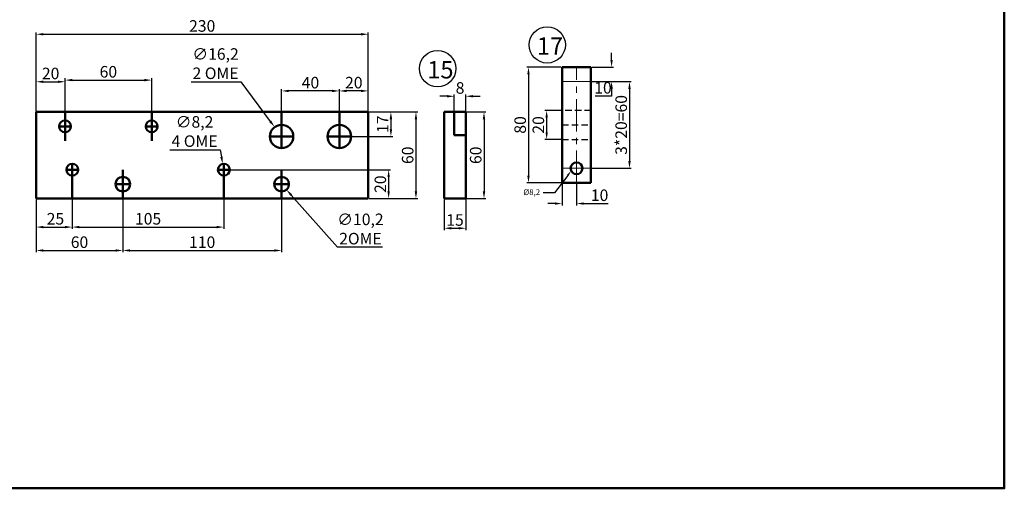
# Model space of a CAD drawing. Units: millimetres. Extents: x -749 to 333, y -22 to 680.
# Tile 3 of 4: x -349 to 333, y -22 to 302. Entities that reach past the tile are written whole.
import ezdxf
from ezdxf import colors
from ezdxf.entities.mleader import LeaderData, LeaderLine
from ezdxf.math import Vec2, Vec3

# ---------------------------------------------------------------- set-up
doc = ezdxf.new("R2010")
doc.units = ezdxf.units.MM
doc.header["$LTSCALE"] = 0.7
doc.linetypes.add('CENTER', pattern=[50.8, 31.75, -6.35, 6.35, -6.35])
doc.linetypes.add('HIDDEN', pattern=[9.525, 6.35, -3.175])
for name, color, linetype, lineweight in [('M-CNTR', 1, 'CENTER', 18), ('M-DIMS', 2, 'Continuous', 25), ('M-HIDN', 4, 'HIDDEN', 25), ('M-OUTL', 7, 'Continuous', 50), ('M-TEXT', 3, 'Continuous', 25), ('M-TTLB', 7, 'Continuous', 50)]:
    doc.layers.add(name, color=color, linetype=linetype, lineweight=lineweight)
doc.styles.get("Standard").update_dxf_attribs({"font": 'arial.ttf'})
doc.dimstyles.new('ISO-25', dxfattribs={"dimtxt": 8, "dimasz": 5, "dimexe": 1.25, "dimexo": 0.625, "dimtad": 1, "dimtoh": 1, "dimtxsty": 'Standard', "dimcen": 2.5, "dimadec": 0, "dimazin": 0, "dimtfac": 1, "dimtofl": 0, "dimtmove": 0, "dimatfit": 3, "dimfxl": 1, "dimarcsym": 0})

# ---------------------------------------------------------------- blocks, each defined once
blk = doc.blocks.new('*D43')
at = {"layer": 'Defpoints', "color": 0, "transparency": 16777216}
for p in [(-107.83, 238.25), (-107.83, 178.25), (-74.76, 178.25)]:
    blk.add_point(p, dxfattribs=at)
at = {"layer": 'M-DIMS', "color": 0, "lineweight": -2, "transparency": 16777216}
for p, q in [((-107.21, 238.25), (-73.51, 238.25)), ((-74.76, 233.25), (-74.76, 183.25)), ((-107.21, 178.25), (-73.51, 178.25))]:
    blk.add_line(p, q, dxfattribs=at)
at = {"layer": 'M-DIMS', "color": 0, "transparency": 16777216}
for points in [[(-75.6, 233.25), (-73.93, 233.25), (-74.76, 238.25)], [(-75.6, 183.25), (-73.93, 183.25), (-74.76, 178.25)]]:
    blk.add_solid(points, dxfattribs=at)
at = {"layer": 'M-DIMS', "color": 0, "transparency": 16777216, "insert": (-79.47, 208.25), "char_height": 8, "attachment_point": 5, "rotation": 90}
blk.add_mtext('60', dxfattribs=at)
blk = doc.blocks.new('*D44')
at = {"layer": 'Defpoints', "color": 0, "transparency": 16777216}
for p in [(-127.83, 238.25), (-127.83, 221.25), (-92.12, 221.25)]:
    blk.add_point(p, dxfattribs=at)
at = {"layer": 'M-DIMS', "color": 0, "lineweight": -2, "transparency": 16777216}
for p, q in [((-127.21, 238.25), (-90.87, 238.25)), ((-92.12, 233.25), (-92.12, 226.25)), ((-127.21, 221.25), (-90.87, 221.25))]:
    blk.add_line(p, q, dxfattribs=at)
at = {"layer": 'M-DIMS', "color": 0, "transparency": 16777216}
for points in [[(-92.95, 233.25), (-91.28, 233.25), (-92.12, 238.25)], [(-92.95, 226.25), (-91.28, 226.25), (-92.12, 221.25)]]:
    blk.add_solid(points, dxfattribs=at)
at = {"layer": 'M-DIMS', "color": 0, "transparency": 16777216, "insert": (-96.76, 229.75), "char_height": 8, "attachment_point": 5, "rotation": 90}
blk.add_mtext('17', dxfattribs=at)
blk = doc.blocks.new('*D45')
at = {"layer": 'Defpoints', "color": 0, "transparency": 16777216}
for p in [(-207.83, 198.25), (-107.83, 178.25), (-93.69, 178.25)]:
    blk.add_point(p, dxfattribs=at)
at = {"layer": 'M-DIMS', "color": 0, "lineweight": -2, "transparency": 16777216}
for p, q in [((-207.21, 198.25), (-92.44, 198.25)), ((-93.69, 193.25), (-93.69, 183.25)), ((-107.21, 178.25), (-92.44, 178.25))]:
    blk.add_line(p, q, dxfattribs=at)
at = {"layer": 'M-DIMS', "color": 0, "transparency": 16777216}
for points in [[(-94.53, 193.25), (-92.86, 193.25), (-93.69, 198.25)], [(-94.53, 183.25), (-92.86, 183.25), (-93.69, 178.25)]]:
    blk.add_solid(points, dxfattribs=at)
at = {"layer": 'M-DIMS', "color": 0, "transparency": 16777216, "insert": (-98.4, 188.25), "char_height": 8, "attachment_point": 5, "rotation": 90}
blk.add_mtext('20', dxfattribs=at)
blk = doc.blocks.new('*D46')
at = {"layer": 'Defpoints', "color": 0, "transparency": 16777216}
for p in [(-337.83, 178.25), (-312.83, 178.25), (-312.83, 158.55)]:
    blk.add_point(p, dxfattribs=at)
at = {"layer": 'M-DIMS', "color": 0, "lineweight": -2, "transparency": 16777216}
for p, q in [((-337.83, 177.62), (-337.83, 157.3)), ((-312.83, 177.62), (-312.83, 157.3)), ((-332.83, 158.55), (-317.83, 158.55))]:
    blk.add_line(p, q, dxfattribs=at)
at = {"layer": 'M-DIMS', "color": 0, "transparency": 16777216}
for points in [[(-332.83, 159.39), (-332.83, 157.72), (-337.83, 158.55)], [(-317.83, 159.39), (-317.83, 157.72), (-312.83, 158.55)]]:
    blk.add_solid(points, dxfattribs=at)
at = {"layer": 'M-DIMS', "color": 0, "transparency": 16777216, "insert": (-324.51, 163.26), "char_height": 8, "attachment_point": 5}
blk.add_mtext('25', dxfattribs=at)
blk = doc.blocks.new('*D47')
at = {"layer": 'Defpoints', "color": 0, "transparency": 16777216}
for p in [(-337.83, 178.25), (-277.83, 178.25), (-277.83, 142.35)]:
    blk.add_point(p, dxfattribs=at)
at = {"layer": 'M-DIMS', "color": 0, "lineweight": -2, "transparency": 16777216}
for p, q in [((-337.83, 177.62), (-337.83, 141.1)), ((-277.83, 177.62), (-277.83, 141.1)), ((-332.83, 142.35), (-282.83, 142.35))]:
    blk.add_line(p, q, dxfattribs=at)
at = {"layer": 'M-DIMS', "color": 0, "transparency": 16777216}
for points in [[(-332.83, 143.18), (-332.83, 141.52), (-337.83, 142.35)], [(-282.83, 143.18), (-282.83, 141.52), (-277.83, 142.35)]]:
    blk.add_solid(points, dxfattribs=at)
at = {"layer": 'M-DIMS', "color": 0, "transparency": 16777216, "insert": (-307.83, 147.06), "char_height": 8, "attachment_point": 5}
blk.add_mtext('60', dxfattribs=at)
blk = doc.blocks.new('*D48')
at = {"layer": 'Defpoints', "color": 0, "transparency": 16777216}
for p in [(-312.83, 178.25), (-207.83, 178.25), (-207.83, 158.55)]:
    blk.add_point(p, dxfattribs=at)
at = {"layer": 'M-DIMS', "color": 0, "lineweight": -2, "transparency": 16777216}
for p, q in [((-312.83, 177.62), (-312.83, 157.3)), ((-207.83, 177.62), (-207.83, 157.3)), ((-307.83, 158.55), (-212.83, 158.55))]:
    blk.add_line(p, q, dxfattribs=at)
at = {"layer": 'M-DIMS', "color": 0, "transparency": 16777216}
for points in [[(-307.83, 159.39), (-307.83, 157.72), (-312.83, 158.55)], [(-212.83, 159.39), (-212.83, 157.72), (-207.83, 158.55)]]:
    blk.add_solid(points, dxfattribs=at)
at = {"layer": 'M-DIMS', "color": 0, "transparency": 16777216, "insert": (-260.33, 163.26), "char_height": 8, "attachment_point": 5}
blk.add_mtext('105', dxfattribs=at)
blk = doc.blocks.new('*D49')
at = {"layer": 'Defpoints', "color": 0, "transparency": 16777216}
for p in [(-277.83, 178.25), (-167.83, 178.25), (-167.83, 142.35)]:
    blk.add_point(p, dxfattribs=at)
at = {"layer": 'M-DIMS', "color": 0, "lineweight": -2, "transparency": 16777216}
for p, q in [((-277.83, 177.62), (-277.83, 141.1)), ((-167.83, 177.62), (-167.83, 141.1)), ((-272.83, 142.35), (-172.83, 142.35))]:
    blk.add_line(p, q, dxfattribs=at)
at = {"layer": 'M-DIMS', "color": 0, "transparency": 16777216}
for points in [[(-272.83, 143.18), (-272.83, 141.52), (-277.83, 142.35)], [(-172.83, 143.18), (-172.83, 141.52), (-167.83, 142.35)]]:
    blk.add_solid(points, dxfattribs=at)
at = {"layer": 'M-DIMS', "color": 0, "transparency": 16777216, "insert": (-222.83, 147.06), "char_height": 8, "attachment_point": 5}
blk.add_mtext('110', dxfattribs=at)
blk = doc.blocks.new('*D50')
at = {"layer": 'Defpoints', "color": 0, "transparency": 16777216}
for p in [(-107.83, 292.04), (-337.83, 238.25), (-107.83, 238.25)]:
    blk.add_point(p, dxfattribs=at)
at = {"layer": 'M-DIMS', "color": 0, "lineweight": -2, "transparency": 16777216}
for p, q in [((-337.83, 238.87), (-337.83, 293.29)), ((-107.83, 238.87), (-107.83, 293.29)), ((-332.83, 292.04), (-112.83, 292.04))]:
    blk.add_line(p, q, dxfattribs=at)
at = {"layer": 'M-DIMS', "color": 0, "transparency": 16777216}
for points in [[(-332.83, 292.88), (-332.83, 291.21), (-337.83, 292.04)], [(-112.83, 292.88), (-112.83, 291.21), (-107.83, 292.04)]]:
    blk.add_solid(points, dxfattribs=at)
at = {"layer": 'M-DIMS', "color": 0, "transparency": 16777216, "insert": (-222.83, 296.76), "char_height": 8, "attachment_point": 5}
blk.add_mtext('230', dxfattribs=at)
blk = doc.blocks.new('*D51')
at = {"layer": 'Defpoints', "color": 0, "transparency": 16777216}
for p in [(-317.83, 259.16), (-337.83, 238.25), (-317.83, 238.25)]:
    blk.add_point(p, dxfattribs=at)
at = {"layer": 'M-DIMS', "color": 0, "lineweight": -2, "transparency": 16777216}
for p, q in [((-337.83, 238.87), (-337.83, 260.41)), ((-317.83, 238.87), (-317.83, 260.41)), ((-332.83, 259.16), (-322.83, 259.16))]:
    blk.add_line(p, q, dxfattribs=at)
at = {"layer": 'M-DIMS', "color": 0, "transparency": 16777216}
for points in [[(-332.83, 259.99), (-332.83, 258.32), (-337.83, 259.16)], [(-322.83, 259.99), (-322.83, 258.32), (-317.83, 259.16)]]:
    blk.add_solid(points, dxfattribs=at)
at = {"layer": 'M-DIMS', "color": 0, "transparency": 16777216, "insert": (-327.83, 263.87), "char_height": 8, "attachment_point": 5}
blk.add_mtext('20', dxfattribs=at)
blk = doc.blocks.new('*D52')
at = {"layer": 'Defpoints', "color": 0, "transparency": 16777216}
for p in [(-257.83, 260.31), (-317.83, 238.25), (-257.83, 238.25)]:
    blk.add_point(p, dxfattribs=at)
at = {"layer": 'M-DIMS', "color": 0, "lineweight": -2, "transparency": 16777216}
for p, q in [((-317.83, 238.87), (-317.83, 261.56)), ((-312.83, 260.31), (-262.83, 260.31)), ((-257.83, 238.87), (-257.83, 261.56))]:
    blk.add_line(p, q, dxfattribs=at)
at = {"layer": 'M-DIMS', "color": 0, "transparency": 16777216}
for points in [[(-312.83, 261.15), (-312.83, 259.48), (-317.83, 260.31)], [(-262.83, 261.15), (-262.83, 259.48), (-257.83, 260.31)]]:
    blk.add_solid(points, dxfattribs=at)
at = {"layer": 'M-DIMS', "color": 0, "transparency": 16777216, "insert": (-287.83, 265.02), "char_height": 8, "attachment_point": 5}
blk.add_mtext('60', dxfattribs=at)
blk = doc.blocks.new('*D53')
at = {"layer": 'Defpoints', "color": 0, "transparency": 16777216}
for p in [(-127.83, 252.81), (-127.83, 238.25), (-107.83, 238.25)]:
    blk.add_point(p, dxfattribs=at)
at = {"layer": 'M-DIMS', "color": 0, "lineweight": -2, "transparency": 16777216}
for p, q in [((-127.83, 238.87), (-127.83, 254.06)), ((-112.83, 252.81), (-122.83, 252.81)), ((-107.83, 238.87), (-107.83, 254.06))]:
    blk.add_line(p, q, dxfattribs=at)
at = {"layer": 'M-DIMS', "color": 0, "transparency": 16777216}
for points in [[(-122.83, 253.64), (-122.83, 251.98), (-127.83, 252.81)], [(-112.83, 253.64), (-112.83, 251.98), (-107.83, 252.81)]]:
    blk.add_solid(points, dxfattribs=at)
at = {"layer": 'M-DIMS', "color": 0, "transparency": 16777216, "insert": (-117.83, 257.52), "char_height": 8, "attachment_point": 5}
blk.add_mtext('20', dxfattribs=at)
blk = doc.blocks.new('*D54')
at = {"layer": 'Defpoints', "color": 0, "transparency": 16777216}
for p in [(-167.83, 252.81), (-167.83, 238.25), (-127.83, 238.25)]:
    blk.add_point(p, dxfattribs=at)
at = {"layer": 'M-DIMS', "color": 0, "lineweight": -2, "transparency": 16777216}
for p, q in [((-167.83, 238.87), (-167.83, 254.06)), ((-132.83, 252.81), (-162.83, 252.81)), ((-127.83, 238.87), (-127.83, 254.06))]:
    blk.add_line(p, q, dxfattribs=at)
at = {"layer": 'M-DIMS', "color": 0, "transparency": 16777216}
for points in [[(-162.83, 253.64), (-162.83, 251.98), (-167.83, 252.81)], [(-132.83, 253.64), (-132.83, 251.98), (-127.83, 252.81)]]:
    blk.add_solid(points, dxfattribs=at)
at = {"layer": 'M-DIMS', "color": 0, "transparency": 16777216, "insert": (-147.83, 257.52), "char_height": 8, "attachment_point": 5}
blk.add_mtext('40', dxfattribs=at)
blk = doc.blocks.new('*D55')
at = {"layer": 'Defpoints', "color": 0, "transparency": 16777216}
for p in [(-171.21, 192.07), (-164.45, 184.43)]:
    blk.add_point(p, dxfattribs=at)
at = {"layer": 'M-DIMS', "color": 0, "lineweight": -2, "transparency": 16777216}
for p, q in [((-170.33, 188.25), (-165.33, 188.25)), ((-167.83, 185.75), (-167.83, 190.75)), ((-129.21, 144.6), (-161.14, 180.69)), ((-97.84, 144.6), (-129.21, 144.6))]:
    blk.add_line(p, q, dxfattribs=at)
at = {"layer": 'M-DIMS', "color": 0, "transparency": 16777216}
blk.add_solid([(-160.52, 181.24), (-161.76, 180.13), (-164.45, 184.43)], dxfattribs=at)
at = {"layer": 'M-DIMS', "color": 0, "transparency": 16777216, "insert": (-113.22, 156.18), "char_height": 8, "attachment_point": 5}
blk.add_mtext('∅10,2\\P2OME', dxfattribs=at)
blk = doc.blocks.new('*D56')
at = {"layer": 'Defpoints', "color": 0, "transparency": 16777216}
for p in [(-208.61, 202.28), (-207.06, 194.22)]:
    blk.add_point(p, dxfattribs=at)
at = {"layer": 'M-DIMS', "color": 0, "lineweight": -2, "transparency": 16777216}
for p, q in [((-245.16, 212.1), (-210.5, 212.1)), ((-210.5, 212.1), (-209.55, 207.19)), ((-210.33, 198.25), (-205.33, 198.25)), ((-207.83, 195.75), (-207.83, 200.75))]:
    blk.add_line(p, q, dxfattribs=at)
at = {"layer": 'M-DIMS', "color": 0, "transparency": 16777216}
blk.add_solid([(-208.73, 207.34), (-210.37, 207.03), (-208.61, 202.28)], dxfattribs=at)
at = {"layer": 'M-DIMS', "color": 0, "transparency": 16777216, "insert": (-228.14, 223.67), "char_height": 8, "attachment_point": 5}
blk.add_mtext('∅8,2\\P4 OME', dxfattribs=at)
blk = doc.blocks.new('*D57')
at = {"layer": 'Defpoints', "color": 0, "transparency": 16777216}
for p in [(-172.67, 227.74), (-162.99, 214.76)]:
    blk.add_point(p, dxfattribs=at)
at = {"layer": 'M-DIMS', "color": 0, "lineweight": -2, "transparency": 16777216}
for p, q in [((-230.51, 259.08), (-196.04, 259.08)), ((-196.04, 259.08), (-175.66, 231.75)), ((-170.33, 221.25), (-165.33, 221.25)), ((-167.83, 218.75), (-167.83, 223.75))]:
    blk.add_line(p, q, dxfattribs=at)
at = {"layer": 'M-DIMS', "color": 0, "transparency": 16777216}
blk.add_solid([(-174.99, 232.25), (-176.33, 231.25), (-172.67, 227.74)], dxfattribs=at)
at = {"layer": 'M-DIMS', "color": 0, "transparency": 16777216, "insert": (-213.59, 270.66), "char_height": 8, "attachment_point": 5}
blk.add_mtext('∅16,2\\P2 OME', dxfattribs=at)
blk = doc.blocks.new('*D58')
at = {"layer": 'Defpoints', "color": 0, "transparency": 16777216}
for p in [(-40.22, 249.12), (-48.22, 237.75), (-40.22, 237.75)]:
    blk.add_point(p, dxfattribs=at)
at = {"layer": 'M-DIMS', "color": 0, "lineweight": -2, "transparency": 16777216}
for p, q in [((-53.22, 249.12), (-58.22, 249.12)), ((-48.22, 238.37), (-48.22, 250.37)), ((-40.22, 238.37), (-40.22, 250.37)), ((-35.22, 249.12), (-30.22, 249.12))]:
    blk.add_line(p, q, dxfattribs=at)
at = {"layer": 'M-DIMS', "color": 0, "transparency": 16777216}
for points in [[(-53.22, 249.95), (-53.22, 248.28), (-48.22, 249.12)], [(-35.22, 249.95), (-35.22, 248.28), (-40.22, 249.12)]]:
    blk.add_solid(points, dxfattribs=at)
at = {"layer": 'M-DIMS', "color": 0, "transparency": 16777216, "insert": (-44.22, 253.83), "char_height": 8, "attachment_point": 5}
blk.add_mtext('8', dxfattribs=at)
blk = doc.blocks.new('*D59')
at = {"layer": 'Defpoints', "color": 0, "transparency": 16777216}
for p in [(-55.22, 178.25), (-40.22, 178.25), (-40.22, 157.73)]:
    blk.add_point(p, dxfattribs=at)
at = {"layer": 'M-DIMS', "color": 0, "lineweight": -2, "transparency": 16777216}
for p, q in [((-55.22, 177.62), (-55.22, 156.48)), ((-40.22, 177.62), (-40.22, 156.48)), ((-50.22, 157.73), (-45.22, 157.73))]:
    blk.add_line(p, q, dxfattribs=at)
at = {"layer": 'M-DIMS', "color": 0, "transparency": 16777216}
for points in [[(-50.22, 158.56), (-50.22, 156.9), (-55.22, 157.73)], [(-45.22, 158.56), (-45.22, 156.9), (-40.22, 157.73)]]:
    blk.add_solid(points, dxfattribs=at)
at = {"layer": 'M-DIMS', "color": 0, "transparency": 16777216, "insert": (-47.72, 162.44), "char_height": 8, "attachment_point": 5}
blk.add_mtext('15', dxfattribs=at)
blk = doc.blocks.new('*D60')
at = {"layer": 'Defpoints', "color": 0, "transparency": 16777216}
for p in [(-55.22, 238.25), (-55.22, 178.25), (-27.62, 178.25)]:
    blk.add_point(p, dxfattribs=at)
at = {"layer": 'M-DIMS', "color": 0, "lineweight": -2, "transparency": 16777216}
for p, q in [((-54.59, 238.25), (-26.37, 238.25)), ((-27.62, 233.25), (-27.62, 183.25)), ((-54.59, 178.25), (-26.37, 178.25))]:
    blk.add_line(p, q, dxfattribs=at)
at = {"layer": 'M-DIMS', "color": 0, "transparency": 16777216}
for points in [[(-28.46, 233.25), (-26.79, 233.25), (-27.62, 238.25)], [(-28.46, 183.25), (-26.79, 183.25), (-27.62, 178.25)]]:
    blk.add_solid(points, dxfattribs=at)
at = {"layer": 'M-DIMS', "color": 0, "transparency": 16777216, "insert": (-32.33, 208.25), "char_height": 8, "attachment_point": 5, "rotation": 90}
blk.add_mtext('60', dxfattribs=at)
blk = doc.blocks.new('*D80')
at = {"layer": 'Defpoints', "color": 0, "transparency": 16777216}
for p in [(46.47, 259.26), (46.47, 199.26), (73.15, 199.26)]:
    blk.add_point(p, dxfattribs=at)
at = {"layer": 'M-DIMS', "color": 0, "lineweight": -2, "transparency": 16777216}
for p, q in [((47.1, 259.26), (74.4, 259.26)), ((73.15, 254.26), (73.15, 204.26)), ((47.1, 199.26), (74.4, 199.26))]:
    blk.add_line(p, q, dxfattribs=at)
at = {"layer": 'M-DIMS', "color": 0, "transparency": 16777216}
for points in [[(72.31, 254.26), (73.98, 254.26), (73.15, 259.26)], [(72.31, 204.26), (73.98, 204.26), (73.15, 199.26)]]:
    blk.add_solid(points, dxfattribs=at)
at = {"layer": 'M-DIMS', "color": 0, "transparency": 16777216, "insert": (68.43, 229.26), "char_height": 8, "attachment_point": 5, "rotation": 90}
blk.add_mtext('3*20=60', dxfattribs=at)
blk = doc.blocks.new('*D81')
at = {"layer": 'Defpoints', "color": 0, "transparency": 16777216}
for p in [(26.47, 189.26), (36.47, 189.26), (36.47, 174.84)]:
    blk.add_point(p, dxfattribs=at)
at = {"layer": 'M-DIMS', "color": 0, "lineweight": -2, "transparency": 16777216}
for p, q in [((26.47, 188.64), (26.47, 173.59)), ((36.47, 188.64), (36.47, 173.59)), ((21.47, 174.84), (16.47, 174.84)), ((41.47, 174.84), (58.4, 174.84))]:
    blk.add_line(p, q, dxfattribs=at)
at = {"layer": 'M-DIMS', "color": 0, "transparency": 16777216}
for points in [[(21.47, 175.67), (21.47, 174.01), (26.47, 174.84)], [(41.47, 175.67), (41.47, 174.01), (36.47, 174.84)]]:
    blk.add_solid(points, dxfattribs=at)
at = {"layer": 'M-DIMS', "color": 0, "transparency": 16777216, "insert": (52.44, 179.55), "char_height": 8, "attachment_point": 5}
blk.add_mtext('10', dxfattribs=at)
blk = doc.blocks.new('*D82')
at = {"layer": 'Defpoints', "color": 0, "transparency": 16777216}
for p in [(26.47, 269.26), (3.18, 189.26), (26.47, 189.26)]:
    blk.add_point(p, dxfattribs=at)
at = {"layer": 'M-DIMS', "color": 0, "lineweight": -2, "transparency": 16777216}
for p, q in [((25.85, 269.26), (1.93, 269.26)), ((3.18, 264.26), (3.18, 194.26)), ((25.85, 189.26), (1.93, 189.26))]:
    blk.add_line(p, q, dxfattribs=at)
at = {"layer": 'M-DIMS', "color": 0, "transparency": 16777216}
for points in [[(2.34, 264.26), (4.01, 264.26), (3.18, 269.26)], [(2.34, 194.26), (4.01, 194.26), (3.18, 189.26)]]:
    blk.add_solid(points, dxfattribs=at)
at = {"layer": 'M-DIMS', "color": 0, "transparency": 16777216, "insert": (-1.53, 229.26), "char_height": 8, "attachment_point": 5, "rotation": 90}
blk.add_mtext('80', dxfattribs=at)
blk = doc.blocks.new('*D89')
at = {"layer": 'Defpoints', "color": 0, "ltscale": 0.7, "transparency": 16777216}
for p in [(46.47, 269.26), (46.47, 259.26), (60.75, 259.26)]:
    blk.add_point(p, dxfattribs=at)
at = {"layer": 'M-DIMS', "color": 0, "lineweight": -2, "ltscale": 0.7, "transparency": 16777216}
for p, q in [((60.75, 274.26), (60.75, 279.26)), ((47.1, 269.26), (62, 269.26)), ((47.1, 259.26), (62, 259.26)), ((60.75, 254.26), (60.75, 249.26)), ((60.75, 249.26), (49.44, 249.26))]:
    blk.add_line(p, q, dxfattribs=at)
at = {"layer": 'M-DIMS', "color": 0, "ltscale": 0.7, "transparency": 16777216}
for points in [[(59.91, 274.26), (61.58, 274.26), (60.75, 269.26)], [(59.91, 254.26), (61.58, 254.26), (60.75, 259.26)]]:
    blk.add_solid(points, dxfattribs=at)
at = {"layer": 'M-DIMS', "color": 0, "ltscale": 0.7, "transparency": 16777216, "insert": (54.78, 253.97), "char_height": 8, "attachment_point": 5}
blk.add_mtext('10', dxfattribs=at)
blk = doc.blocks.new('*D90')
at = {"layer": 'Defpoints', "color": 0, "ltscale": 0.7, "transparency": 16777216}
for p in [(26.47, 239.26), (15.77, 219.26), (26.47, 219.26)]:
    blk.add_point(p, dxfattribs=at)
at = {"layer": 'M-DIMS', "color": 0, "lineweight": -2, "ltscale": 0.7, "transparency": 16777216}
for p, q in [((25.85, 239.26), (14.52, 239.26)), ((15.77, 234.26), (15.77, 224.26)), ((25.85, 219.26), (14.52, 219.26))]:
    blk.add_line(p, q, dxfattribs=at)
at = {"layer": 'M-DIMS', "color": 0, "ltscale": 0.7, "transparency": 16777216}
for points in [[(14.93, 234.26), (16.6, 234.26), (15.77, 239.26)], [(14.93, 224.26), (16.6, 224.26), (15.77, 219.26)]]:
    blk.add_solid(points, dxfattribs=at)
at = {"layer": 'M-DIMS', "color": 0, "ltscale": 0.7, "transparency": 16777216, "insert": (11.06, 229.26), "char_height": 8, "attachment_point": 5, "rotation": 90}
blk.add_mtext('20', dxfattribs=at)
blk = doc.blocks.new('HOLE-8')
blk.add_line((0, 4.1), (8.2, 4.1))
blk.add_circle((4.1, 4.1), 4.1)
blk = doc.blocks.new('HOLE-10')
blk.add_line((10.2, 5.1), (0, 5.1))
blk.add_circle((5.1, 5.1), 5.1)
blk = doc.blocks.new('HOLE-16')
blk.add_line((0, 8.1), (16.2, 8.1))
blk.add_circle((8.1, 8.1), 8.1)

msp = doc.modelspace()

# ---------------------------------------------------------------- linework, layer by layer
at = {"layer": 'M-CNTR'}
for p, q in [((36.471, 189.261), (36.471, 269.261)), ((46.471, 259.261), (26.471, 259.261)), ((26.471, 199.261), (46.471, 199.261))]:
    msp.add_line(p, q, dxfattribs=at)
at = {"layer": 'M-HIDN'}
for p, q in [((46.471, 239.261), (26.471, 239.261)), ((26.471, 229.261), (46.471, 229.261)), ((26.471, 219.261), (46.471, 219.261))]:
    msp.add_line(p, q, dxfattribs=at)
at = {"layer": 'M-OUTL'}
for p, q in [((26.471, 269.261), (26.471, 189.261)), ((46.471, 269.261), (26.471, 269.261)), ((46.471, 189.261), (46.471, 269.261)), ((-337.833, 238.25), (-107.833, 238.25)), ((-337.833, 178.25), (-337.833, 238.25)), ((-317.833, 218.25), (-317.833, 238.25)), ((-257.833, 218.25), (-257.833, 238.25)), ((-167.833, 238.25), (-167.833, 213.15)), ((-127.833, 238.25), (-127.833, 213.15)), ((-107.833, 238.25), (-107.833, 178.25)), ((-55.22, 238.25), (-55.22, 178.25)), ((-40.22, 238.25), (-55.22, 238.25)), ((-48.22, 222.104), (-48.22, 238.25)), ((-40.22, 178.25), (-40.22, 238.25)), ((-40.22, 222.104), (-48.22, 222.104)), ((-312.833, 178.25), (-312.833, 202.35)), ((-277.833, 178.25), (-277.833, 198.25)), ((-207.833, 178.25), (-207.833, 202.35)), ((-167.833, 178.25), (-167.833, 198.25)), ((-167.833, 193.35), (-167.833, 178.25)), ((26.471, 189.261), (46.471, 189.261)), ((-107.833, 178.25), (-337.833, 178.25)), ((-55.22, 178.25), (-40.22, 178.25))]:
    msp.add_line(p, q, dxfattribs=at)
msp.add_circle((36.471, 199.261), 4.1, dxfattribs=at)
at = {"layer": 'M-TEXT'}
for centre in [(16.159, 284.695), (-59.785, 268.242)]:
    msp.add_circle(centre, 12.598, dxfattribs=at)
at = {"layer": 'M-TTLB', "ltscale": 0.7}
msp.add_lwpolyline([(-749.362, 679.91), (332.782, 679.91), (332.782, -22.287), (-749.362, -22.287)], close=True, dxfattribs=at)

# ---------------------------------------------------------------- block references
at = {"layer": 'M-OUTL'}
for name, p in [('HOLE-8', (-321.933, 224.149)), ('HOLE-8', (-261.933, 224.149)), ('HOLE-16', (-175.933, 213.15)), ('HOLE-16', (-135.933, 213.15)), ('HOLE-10', (-282.933, 183.15)), ('HOLE-10', (-172.933, 183.15))]:
    msp.add_blockref(name, p, dxfattribs=at)
at = {"layer": 'M-OUTL', "rotation": 180}
for p in [(-308.734, 202.35), (-203.734, 202.35)]:
    msp.add_blockref('HOLE-8', p, dxfattribs=at)

# ---------------------------------------------------------------- texts
at = {"layer": 'M-TEXT', "char_height": 12, "attachment_point": 1}
for s, insert in [('\\pxql;17', (9.013, 289.914)), ('\\pxql;15', (-66.932, 273.461))]:
    msp.add_mtext_dynamic_manual_height_columns(s, width=30.10277, gutter_width=12.5, heights=[0], dxfattribs=dict(at, insert=insert))

# ---------------------------------------------------------------- dimensions: what is measured, and where the dimension line sits
at = {"layer": 'M-DIMS'}
for base, p1, p2, picture, middle in [((-107.833, 292.044), (-337.833, 238.25), (-107.833, 238.25), '*D50', (-222.833, 296.756)), ((-317.833, 259.158), (-337.833, 238.25), (-317.833, 238.25), '*D51', (-327.833, 263.867)), ((-257.833, 260.312), (-317.833, 238.25), (-257.833, 238.25), '*D52', (-287.833, 265.021)), ((-167.833, 252.811), (-127.833, 238.25), (-167.833, 238.25), '*D54', (-147.833, 257.521)), ((-127.833, 252.811), (-107.833, 238.25), (-127.833, 238.25), '*D53', (-117.833, 257.521)), ((-40.22, 249.117), (-48.22, 237.75), (-40.22, 237.75), '*D58', (-44.22, 253.827)), ((36.471, 174.841), (26.471, 189.261), (36.471, 189.261), '*D81', (52.435, 179.55)), ((-277.833, 142.349), (-337.833, 178.25), (-277.833, 178.25), '*D47', (-307.833, 147.059)), ((-207.833, 158.554), (-312.833, 178.25), (-207.833, 178.25), '*D48', (-260.333, 163.263)), ((-167.833, 142.349), (-277.833, 178.25), (-167.833, 178.25), '*D49', (-222.833, 147.059)), ((-40.22, 157.73), (-55.22, 178.25), (-40.22, 178.25), '*D59', (-47.72, 162.44))]:
    dim = msp.add_linear_dim(base=base, p1=p1, p2=p2, dimstyle='ISO-25', override={"dimclrd": 0, "dimclre": 0, "dimclrt": 0}, dxfattribs=at)
    dim.commit()
    dim.dimension.update_dxf_attribs({"geometry": picture, "text_midpoint": middle})
for p1, p2, text, picture, middle in [((-162.992, 214.756), (-172.674, 227.744), '<>\\P2 OME', '*D57', (-213.587, 259.084)), ((-171.213, 192.069), (-164.454, 184.43), '<>\\P2OME', '*D55', (-113.216, 144.603))]:
    dim = msp.add_diameter_dim_2p(p1=p1, p2=p2, text=text, dimstyle='ISO-25', override={"dimclrd": 0, "dimclre": 0, "dimclrt": 0}, dxfattribs=at)
    dim.commit()
    dim.dimension.update_dxf_attribs({"geometry": picture, "text_midpoint": middle, "dimtype": 163})
at = {"layer": 'M-DIMS', "ltscale": 0.7}
dim = msp.add_linear_dim(base=(60.746, 259.261), p1=(46.471, 269.261), p2=(46.471, 259.261), angle=90, dimstyle='ISO-25', override={"dimclrd": 0, "dimclre": 0, "dimclrt": 0}, dxfattribs=at)
dim.commit()
dim.dimension.update_dxf_attribs({"geometry": '*D89', "text_midpoint": (54.781, 253.971)})
at = {"layer": 'M-DIMS'}
dim = msp.add_linear_dim(base=(3.178, 189.261), p1=(26.471, 269.261), p2=(26.471, 189.261), angle=90, dimstyle='ISO-25', override={"dimclrd": 0, "dimclre": 0, "dimclrt": 0}, dxfattribs=at)
dim.commit()
dim.dimension.update_dxf_attribs({"geometry": '*D82', "text_midpoint": (3.178, 229.261), "dimtype": 160})
dim = msp.add_linear_dim(base=(73.146, 199.261), p1=(46.471, 259.261), p2=(46.471, 199.261), angle=90, text='3*20=<>', dimstyle='ISO-25', override={"dimclrd": 0, "dimclre": 0, "dimclrt": 0}, dxfattribs=at)
dim.commit()
dim.dimension.update_dxf_attribs({"geometry": '*D80', "text_midpoint": (68.433, 229.261)})
dim = msp.add_diameter_dim_2p(p1=(-207.059, 194.223), p2=(-208.607, 202.276), text='<>\\P4 OME', dimstyle='ISO-25', override={"dimclrd": 0, "dimclre": 0, "dimclrt": 0}, dxfattribs=at)
dim.commit()
dim.dimension.update_dxf_attribs({"geometry": '*D56', "text_midpoint": (-228.138, 223.674)})
at = {"layer": 'M-DIMS', "ltscale": 0.7}
dim = msp.add_linear_dim(base=(15.768, 219.261), p1=(26.471, 239.261), p2=(26.471, 219.261), angle=90, dimstyle='ISO-25', override={"dimclrd": 0, "dimclre": 0, "dimclrt": 0}, dxfattribs=at)
dim.commit()
dim.dimension.update_dxf_attribs({"geometry": '*D90', "text_midpoint": (15.768, 229.261), "dimtype": 160})
at = {"layer": 'M-DIMS'}
for base, p1, p2, picture, middle in [((-92.117, 221.25), (-127.833, 238.25), (-127.833, 221.25), '*D44', (-96.758, 229.75)), ((-74.765, 178.25), (-107.833, 238.25), (-107.833, 178.25), '*D43', (-79.474, 208.25)), ((-27.624, 178.25), (-55.22, 238.25), (-55.22, 178.25), '*D60', (-32.334, 208.25)), ((-93.694, 178.25), (-207.833, 198.25), (-107.833, 178.25), '*D45', (-98.404, 188.25))]:
    dim = msp.add_linear_dim(base=base, p1=p1, p2=p2, angle=90, dimstyle='ISO-25', override={"dimclrd": 0, "dimclre": 0, "dimclrt": 0}, dxfattribs=at)
    dim.commit()
    dim.dimension.update_dxf_attribs({"geometry": picture, "text_midpoint": middle})
dim = msp.add_linear_dim(base=(-312.833, 158.554), p1=(-337.833, 178.25), p2=(-312.833, 178.25), dimstyle='ISO-25', override={"dimclrd": 0, "dimclre": 0, "dimclrt": 0}, dxfattribs=at)
dim.commit()
dim.dimension.update_dxf_attribs({"geometry": '*D46', "text_midpoint": (-324.506, 158.554), "dimtype": 160})

# ---------------------------------------------------------------- leaders
at = {"layer": 'M-TEXT', "ltscale": 0.7}
ml = msp.add_multileader_mtext('Standard', dxfattribs=at)
ml.set_content('%%C8,2', color=256)
ml.set_leader_properties()
ml.build(insert=Vec2(0, 0))
ctx = ml.context
ctx.base_point, ctx.plane_origin = Vec3(-2.35, 182.342), Vec3(32.766, 197.506)
ctx.text_align_type = 2
notes = []
notes.append((ctx, [(0, (1, 1, 0), (21.243, 182.342), (-1, 0), 8, [(0, [(32.766, 197.506)], 0, [])])]))
ctx.mtext.insert, ctx.mtext.alignment, ctx.mtext.flow_direction = Vec3(11.243, 184.738), 3, 5
for ctx, leaders in notes:
    for number, flags, end, landing, length, lines in leaders:
        leader = LeaderData()
        leader.index, (leader.has_last_leader_line, leader.has_dogleg_vector, leader.attachment_direction) = number, flags
        leader.last_leader_point, leader.dogleg_vector, leader.dogleg_length = Vec3(end), Vec3(landing), length
        for number, points, colour, breaks in lines:
            line = LeaderLine()
            line.index, line.vertices, line.color, line.breaks = number, Vec3.list(points), colors.encode_raw_color(colour), breaks
            leader.lines.append(line)
        ctx.leaders.append(leader)

doc.saveas('drawing.dxf')
